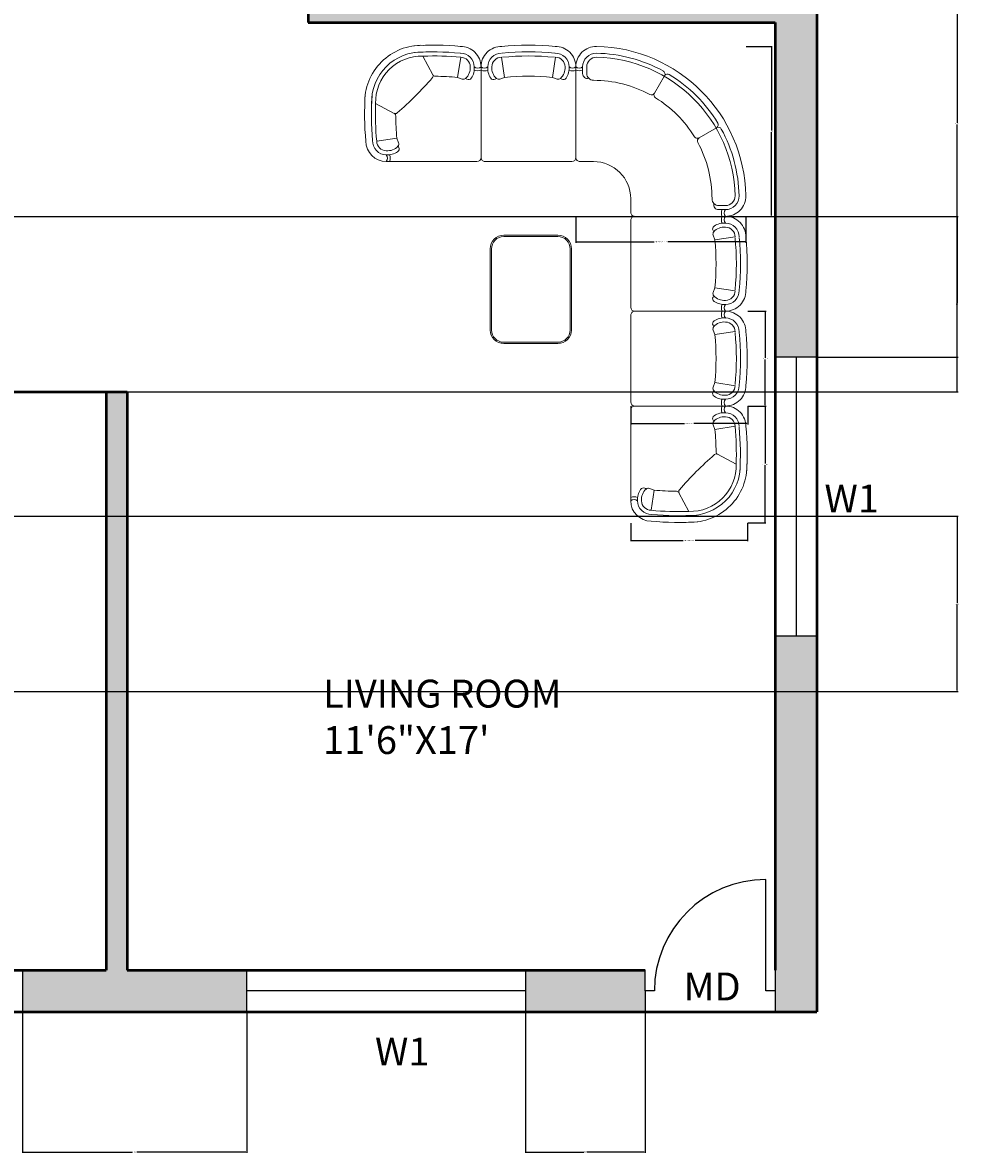
# Model space of a CAD drawing. Units: inches. Extents: x -15 to 420, y -514 to 86.
# Tile 3 of 8: x 218 to 420, y -494 to -251. Entities that reach past the tile are written whole.
import ezdxf

# ---------------------------------------------------------------- set-up
doc = ezdxf.new("R2010")
doc.units = ezdxf.units.IN
doc.header["$MEASUREMENT"] = 0
for name, color, linetype, lineweight in [('A-ANNO-DIMS', 2, 'Continuous', 18), ('A-ANNO-TEXT', 7, 'Continuous', 18), ('A-AREA-IDEN', 7, 'Continuous', 25), ('A-DOOR', 4, 'Continuous', 25), ('A-FURN', 8, 'Continuous', 18), ('A-GLAZ', 41, 'Continuous', 25), ('A-WALL', 7, 'Continuous', 50), ('A-WALL-PATT', 8, 'Continuous', 13)]:
    doc.layers.add(name, color=color, linetype=linetype, lineweight=lineweight)
doc.styles.get("Standard").update_dxf_attribs({"font": 'arial.ttf'})
doc.dimstyles.get("Standard").update_dxf_attribs({"dimtxt": 0.18, "dimasz": 0.18, "dimexe": 0.18, "dimexo": 0.0625, "dimgap": 0.09, "dimtad": 0, "dimtih": 1, "dimtoh": 1, "dimdec": 0, "dimzin": 0, "dimdsep": 46, "dimlunit": 3, "dimtxsty": 'Standard', "dimcen": 0.09, "dimadec": 0, "dimazin": 0, "dimtfac": 1, "dimtdec": 0, "dimtofl": 0, "dimtmove": 0, "dimatfit": 3, "dimfxl": 1, "dimtolj": 1, "dimtzin": 0, "dimarcsym": 0})

# ---------------------------------------------------------------- blocks, each defined once
blk = doc.blocks.new('A$C707258B2')
at = {"color": 0}
for p, q in [((0.4042, 0.342), (1.0739, 0.342)), ((0.4042, 0.292), (0.4544, 0.292)), ((0.4042, 0.262), (0.4539, 0.262)), ((1.1039, 0.312), (1.1039, 0.212)), ((1.4789, -0.063), (1.3789, -0.063)), ((1.5089, -0.7628), (1.5089, -0.093)), ((0.5998, -0.2378), (0.4699, -0.3128)), ((0.9291, -0.5671), (0.8541, -0.697)), ((1.4289, -0.7628), (1.4289, -0.713)), ((1.4589, -0.7628), (1.4589, -0.7125))]:
    blk.add_line(p, q, dxfattribs=at)
for centre, radius, start, end in [((0.4042, 0.192), 0.15, 90, 181.17538), ((0.3779, 0.317), 0.0362, 316.39718, 43.60282), ((0.3679, 0.317), 0.0662, 337.82984, 22.17016), ((1.0739, 0.312), 0.03, 360, 90), ((0.4042, 0.192), 0.1, 90, 181.17538), ((0.4042, 0.192), 0.07, 90, 181.17538), ((0.4539, 0.212), 0.05, 360, 90), ((0.4548, 0.2564), 0.0357, 345.42616, 90.55549), ((1.3789, 0.212), 1.125, 181.17538, 268.82462), ((1.3789, 0.212), 1.075, 181.17538, 208.63569), ((1.3789, 0.212), 1.045, 181.17538, 268.82462), ((1.3789, 0.212), 0.875, 180, 208.40825), ((1.3789, 0.212), 0.275, 180, 270), ((1.4789, -0.093), 0.03, 360, 90), ((0.5873, -0.2162), 0.025, 300, 28.40825), ((0.6123, -0.2595), 0.025, 31.59175, 120), ((1.3789, 0.212), 0.875, 211.59175, 238.40825), ((0.4574, -0.2912), 0.025, 208.63569, 300), ((0.4824, -0.3345), 0.025, 120, 211.36431), ((1.3789, 0.212), 1.075, 211.36431, 238.63569), ((0.9075, -0.5546), 0.025, 330, 58.40825), ((0.9508, -0.5796), 0.025, 61.59175, 150), ((1.3789, 0.212), 0.875, 241.59175, 270), ((1.3789, -0.713), 0.05, 360, 90), ((0.8324, -0.6845), 0.025, 238.63569, 330), ((0.8757, -0.7095), 0.025, 150, 241.36431), ((1.3789, 0.212), 1.075, 241.36431, 268.82462), ((1.4255, -0.7093), 0.0336, 354.63008, 109.38826), ((1.4839, -0.7988), 0.0662, 67.82984, 112.17016), ((1.3589, -0.7628), 0.15, 268.82462, 360), ((1.3589, -0.7628), 0.1, 268.82462, 360), ((1.3589, -0.7628), 0.07, 268.82462, 360), ((1.4839, -0.789), 0.0362, 46.39718, 133.60282)]:
    blk.add_arc(centre, radius, start, end, dxfattribs=at)
blk = doc.blocks.new('part 01')
at = {"color": 0}
for p, q in [((-669.8, 700), (0, 700)), ((30, 30), (30, 670)), ((-590.9, 527.1), (-739.8, 550)), ((-590.9, 527.1), (-578.5, 561.2)), ((-590.9, 172.9), (-739.8, 150)), ((-590.9, 172.9), (-578.5, 138.8)), ((-669.8, 0), (0, 0))]:
    blk.add_line(p, q, dxfattribs=at)
for centre, radius, start, end in [((-669.8, 550), 150, 90, 181.17538), ((-696, 675), 36.2, 316.39718, 43.60282), ((-705.9, 675), 66.2, 337.82984, 22.17016), ((0, 670), 30, 0, 90), ((-669.8, 550), 100, 90, 181.17538), ((-669.8, 550), 70, 90, 181.17538), ((-659.7, 517.8), 132.7, 56.08973, 95.61316), ((-659.7, 517.8), 102.7, 42.00663, 95.61316), ((-599.7, 607.2), 25, 332.96082, 56.08973), ((-624.8, 620), 53.2, 321.00172, 332.96082), ((-602, 569.8), 25, 340, 42.00663), ((1178.1, 350), 2007.9, 174.28354, 185.71646), ((1178.1, 350), 1957.9, 174.28354, 185.71646), ((1178.1, 350), 1927.9, 174.28354, 185.71646), ((1178.1, 350), 1777.9, 174.28354, 185.71646), ((-669.8, 150), 150, 178.82462, 270), ((-669.8, 150), 100, 178.82462, 270), ((-669.8, 150), 70, 178.82462, 270), ((-659.7, 182.2), 102.7, 264.38684, 317.99337), ((-599.7, 92.8), 25, 303.91027, 27.03918), ((-602, 130.2), 25, 317.99337, 20), ((-624.8, 80), 53.2, 27.03918, 38.99828), ((-659.7, 182.2), 132.7, 264.38684, 303.91027), ((-696, 25), 36.2, 316.39718, 43.60282), ((-705.9, 25), 66.2, 337.82984, 22.17016), ((0, 30), 30, 270, 0)]:
    blk.add_arc(centre, radius, start, end, dxfattribs=at)
blk = doc.blocks.new('part02')
at = {"color": 0}
for p, q in [((0, -669.8), (0, 0)), ((30, 30), (699.8, 30)), ((620.9, -142.9), (608.5, -108.8)), ((620.9, -142.9), (769.8, -120)), ((640.4, -325.6), (778.2, -398.9)), ((172.9, -590.9), (138.8, -578.5)), ((172.9, -590.9), (150, -739.8)), ((355.6, -610.4), (428.9, -748.2))]:
    blk.add_line(p, q, dxfattribs=at)
for centre, radius, start, end in [((30, 0), 30, 90, 180), ((726, 5), 56.2, 153.6122, 206.66656), ((726, 5), 36.2, 136.39718, 223.60282), ((699.8, -120), 150, 0, 90), ((629.7, -62.8), 25, 123.91027, 207.03918), ((632, -100.2), 25, 137.99337, 200), ((654.8, -50), 53.2, 207.03918, 218.99828), ((689.7, -152.2), 102.7, 84.38684, 137.99337), ((689.3, -151.3), 131.7, 85.43775, 123.98866), ((699.5, -120.6), 100.6, 357.50055, 89.85796), ((699.8, -120), 70, 0, 90), ((-1148.1, -320), 1777.9, 0.38365, 5.71646), ((-1228.2, -319.5), 2007.9, 357.73494, 5.70316), ((-1148.1, -320), 1957.9, 355.86566, 5.71646), ((-1148.1, -320), 2007.9, 355.81801, 5.71646), ((2219.8, -2189.8), 2454.4, 130.6961, 139.3039), ((632.4, -344.1), 20, 62, 130.6961), ((649.7, -308), 20, 180.38365, 242), ((439.4, -409.4), 418.9, 268.21809, 1.78191), ((439.4, -409.4), 368.9, 268.21809, 1.78191), ((439.4, -409.4), 338.9, 268.21809, 1.78191), ((92.8, -599.7), 25, 62.96082, 146.08973), ((182.2, -659.7), 102.7, 132.00663, 185.61316), ((80, -624.8), 53.2, 51.00172, 62.96082), ((130.2, -602), 25, 70, 132.00663), ((25, -696), 56.2, 63.33344, 116.3878), ((25, -696), 36.2, 46.39718, 133.60282), ((182.2, -659.7), 132.7, 146.08973, 185.61316), ((350, 1178.1), 1777.9, 264.28354, 269.61635), ((338, -619.7), 20, 28, 89.61635), ((374.1, -602.4), 20, 139.3039, 208), ((150, -669.8), 150, 180, 271.17538), ((150, -669.8), 100, 180, 271.17538), ((150, -669.8), 70, 180, 270), ((349.5, 1258.2), 2007.9, 264.29684, 272.26506), ((350, 1178.1), 2007.9, 264.28354, 274.18199), ((350, 1178.1), 1957.9, 264.28354, 274.13434)]:
    blk.add_arc(centre, radius, start, end, dxfattribs=at)
blk = doc.blocks.new('DOOR-SWING-24IN')
for p, q in [((26, 0), (26, 24)), ((2, 0), (0, 0)), ((28, 0), (26, 0))]:
    blk.add_line(p, q)
blk.add_arc((26, 0), 24, 90, 180)
blk = doc.blocks.new('WIN-W1-60IN')
for p, q in [((0, 60), (0, 0)), ((4.5, 60), (4.5, 0)), ((9, 0), (9, 60))]:
    blk.add_line(p, q)
blk = doc.blocks.new('*D25')
at = {"layer": 'A-ANNO-DIMS', "color": 0, "lineweight": -2, "transparency": 16777216}
for p, q in [((349.34, -333.49), (349.34, -337.38)), ((374.51, -333.49), (374.51, -337.38)), ((349.52, -337.2), (360.92, -337.2)), ((374.33, -337.2), (362.92, -337.2))]:
    blk.add_line(p, q, dxfattribs=at)
at = {"layer": 'A-ANNO-DIMS', "color": 0, "transparency": 16777216}
for points in [[(349.52, -337.17), (349.52, -337.23), (349.34, -337.2)], [(374.33, -337.17), (374.33, -337.23), (374.51, -337.2)]]:
    blk.add_solid(points, dxfattribs=at)
at = {"layer": 'Defpoints', "color": 0, "transparency": 16777216}
for p in [(349.34, -333.43), (374.51, -333.43), (349.34, -337.2)]:
    blk.add_point(p, dxfattribs=at)
at = {"layer": 'A-ANNO-DIMS', "color": 0, "transparency": 16777216, "insert": (361.92, -337.2), "char_height": 0.18, "attachment_point": 5}
blk.add_mtext('\\A1;SEAT 2\'-1" TYP.', dxfattribs=at)
blk = doc.blocks.new('*D26')
at = {"layer": 'A-ANNO-DIMS', "color": 0, "lineweight": -2, "transparency": 16777216}
for p, q in [((374.57, -313.02), (378.46, -313.02)), ((378.28, -313.2), (378.28, -323.04)), ((378.28, -333.25), (378.28, -323.41)), ((374.57, -333.43), (378.46, -333.43))]:
    blk.add_line(p, q, dxfattribs=at)
at = {"layer": 'A-ANNO-DIMS', "color": 0, "transparency": 16777216}
for points in [[(378.25, -313.2), (378.31, -313.2), (378.28, -313.02)], [(378.25, -333.25), (378.31, -333.25), (378.28, -333.43)]]:
    blk.add_solid(points, dxfattribs=at)
at = {"layer": 'Defpoints', "color": 0, "transparency": 16777216}
for p in [(374.51, -313.02), (374.51, -333.43), (378.28, -333.43)]:
    blk.add_point(p, dxfattribs=at)
at = {"layer": 'A-ANNO-DIMS', "color": 0, "transparency": 16777216, "insert": (378.28, -323.22), "char_height": 0.18, "attachment_point": 5}
blk.add_mtext('\\A1;1\'-8 1/2" TYP.', dxfattribs=at)
blk = doc.blocks.new('*D27')
at = {"layer": 'A-ANNO-DIMS', "color": 0, "lineweight": -2, "transparency": 16777216}
for p, q in [((349.34, -358.65), (349.34, -362.55)), ((374.5, -358.65), (374.5, -362.55)), ((349.52, -362.37), (360.62, -362.37)), ((374.32, -362.37), (363.21, -362.37))]:
    blk.add_line(p, q, dxfattribs=at)
at = {"layer": 'A-ANNO-DIMS', "color": 0, "transparency": 16777216}
for points in [[(349.52, -362.34), (349.52, -362.4), (349.34, -362.37)], [(374.32, -362.34), (374.32, -362.4), (374.5, -362.37)]]:
    blk.add_solid(points, dxfattribs=at)
at = {"layer": 'Defpoints', "color": 0, "transparency": 16777216}
for p in [(349.34, -358.59), (374.5, -358.59), (349.34, -362.37)]:
    blk.add_point(p, dxfattribs=at)
at = {"layer": 'A-ANNO-DIMS', "color": 0, "transparency": 16777216, "insert": (361.92, -362.37), "char_height": 0.18, "attachment_point": 5}
blk.add_mtext('\\A1;END SEAT 2\'-1" TYP.', dxfattribs=at)
blk = doc.blocks.new('*D28')
at = {"layer": 'A-ANNO-DIMS', "color": 0, "lineweight": -2, "transparency": 16777216}
for p, q in [((374.56, -333.43), (378.45, -333.43)), ((378.27, -333.61), (378.27, -345.83)), ((378.27, -358.41), (378.27, -346.19)), ((374.56, -358.59), (378.45, -358.59))]:
    blk.add_line(p, q, dxfattribs=at)
at = {"layer": 'A-ANNO-DIMS', "color": 0, "transparency": 16777216}
for points in [[(378.24, -333.61), (378.3, -333.61), (378.27, -333.43)], [(378.24, -358.41), (378.3, -358.41), (378.27, -358.59)]]:
    blk.add_solid(points, dxfattribs=at)
at = {"layer": 'Defpoints', "color": 0, "transparency": 16777216}
for p in [(374.5, -333.43), (374.5, -358.59), (378.27, -358.59)]:
    blk.add_point(p, dxfattribs=at)
at = {"layer": 'A-ANNO-DIMS', "color": 0, "transparency": 16777216, "insert": (378.27, -346.01), "char_height": 0.18, "attachment_point": 5}
blk.add_mtext('\\A1;2\'-1" TYP.', dxfattribs=at)
blk = doc.blocks.new('*D29')
at = {"layer": 'A-ANNO-DIMS', "color": 0, "lineweight": -2, "transparency": 16777216}
for p, q in [((337.52, -292.66), (337.52, -298.27)), ((374.14, -292.66), (374.14, -298.27)), ((337.7, -298.09), (354.35, -298.09)), ((373.96, -298.09), (357.31, -298.09))]:
    blk.add_line(p, q, dxfattribs=at)
at = {"layer": 'A-ANNO-DIMS', "color": 0, "transparency": 16777216}
for points in [[(337.7, -298.06), (337.7, -298.12), (337.52, -298.09)], [(373.96, -298.06), (373.96, -298.12), (374.14, -298.09)]]:
    blk.add_solid(points, dxfattribs=at)
at = {"layer": 'Defpoints', "color": 0, "transparency": 16777216}
for p in [(337.52, -292.6), (374.14, -292.6), (337.52, -298.09)]:
    blk.add_point(p, dxfattribs=at)
at = {"layer": 'A-ANNO-DIMS', "color": 0, "transparency": 16777216, "insert": (355.83, -298.09), "char_height": 0.18, "attachment_point": 5}
blk.add_mtext('\\A1;CORNER SEAT 3\'-0 1/2"', dxfattribs=at)
blk = doc.blocks.new('*D30')
at = {"layer": 'A-ANNO-DIMS', "color": 0, "lineweight": -2, "transparency": 16777216}
for p, q in [((374.2, -255.99), (379.81, -255.99)), ((379.63, -256.17), (379.63, -274.11)), ((379.63, -292.42), (379.63, -274.48)), ((374.2, -292.6), (379.81, -292.6))]:
    blk.add_line(p, q, dxfattribs=at)
at = {"layer": 'A-ANNO-DIMS', "color": 0, "transparency": 16777216}
for points in [[(379.6, -256.17), (379.66, -256.17), (379.63, -255.99)], [(379.6, -292.42), (379.66, -292.42), (379.63, -292.6)]]:
    blk.add_solid(points, dxfattribs=at)
at = {"layer": 'Defpoints', "color": 0, "transparency": 16777216}
for p in [(374.14, -255.99), (374.14, -292.6), (379.63, -292.6)]:
    blk.add_point(p, dxfattribs=at)
at = {"layer": 'A-ANNO-DIMS', "color": 0, "transparency": 16777216, "insert": (379.63, -274.29), "char_height": 0.18, "attachment_point": 5}
blk.add_mtext('\\A1;3\'-0 1/2"', dxfattribs=at)
blk = doc.blocks.new('*D47')
at = {"layer": 'A-ANNO-DIMS', "color": 0, "lineweight": -2, "transparency": 16777216}
for p, q in [((164.57, -292.63), (419.8, -292.63)), ((419.62, -292.81), (419.62, -311.32)), ((419.62, -330.2), (419.62, -311.69)), ((164.57, -330.38), (419.8, -330.38))]:
    blk.add_line(p, q, dxfattribs=at)
at = {"layer": 'A-ANNO-DIMS', "color": 0, "transparency": 16777216}
for points in [[(419.59, -292.81), (419.65, -292.81), (419.62, -292.63)], [(419.59, -330.2), (419.65, -330.2), (419.62, -330.38)]]:
    blk.add_solid(points, dxfattribs=at)
at = {"layer": 'Defpoints', "color": 0, "transparency": 16777216}
for p in [(164.51, -292.63), (164.51, -330.38), (419.62, -330.38)]:
    blk.add_point(p, dxfattribs=at)
at = {"layer": 'A-ANNO-DIMS', "color": 0, "transparency": 16777216, "insert": (419.62, -311.5), "char_height": 0.18, "attachment_point": 5}
blk.add_mtext('\\A1;3\'-2"', dxfattribs=at)
blk = doc.blocks.new('*D52')
at = {"layer": 'A-ANNO-DIMS', "color": 0, "lineweight": -2, "transparency": 16777216}
for p, q in [((140.49, -357.15), (419.8, -357.15)), ((419.62, -357.33), (419.62, -375.83)), ((419.62, -394.7), (419.62, -376.2)), ((140.49, -394.88), (419.8, -394.88))]:
    blk.add_line(p, q, dxfattribs=at)
at = {"layer": 'A-ANNO-DIMS', "color": 0, "transparency": 16777216}
for points in [[(419.59, -357.33), (419.65, -357.33), (419.62, -357.15)], [(419.59, -394.7), (419.65, -394.7), (419.62, -394.88)]]:
    blk.add_solid(points, dxfattribs=at)
at = {"layer": 'Defpoints', "color": 0, "transparency": 16777216}
for p in [(140.42, -357.15), (140.42, -394.88), (419.62, -394.88)]:
    blk.add_point(p, dxfattribs=at)
at = {"layer": 'A-ANNO-DIMS', "color": 0, "transparency": 16777216, "insert": (419.62, -376.01), "char_height": 0.18, "attachment_point": 5}
blk.add_mtext('\\A1;3\'-1 1/2"', dxfattribs=at)
blk = doc.blocks.new('*D62')
at = {"layer": 'A-ANNO-DIMS', "color": 0, "lineweight": -2, "transparency": 16777216}
for p, q in [((389.49, -222.38), (419.8, -222.38)), ((419.62, -222.56), (419.62, -272.45)), ((419.62, -322.7), (419.62, -272.81)), ((389.49, -322.88), (419.8, -322.88))]:
    blk.add_line(p, q, dxfattribs=at)
at = {"layer": 'A-ANNO-DIMS', "color": 0, "transparency": 16777216}
for points in [[(419.59, -222.56), (419.65, -222.56), (419.62, -222.38)], [(419.59, -322.7), (419.65, -322.7), (419.62, -322.88)]]:
    blk.add_solid(points, dxfattribs=at)
at = {"layer": 'Defpoints', "color": 0, "transparency": 16777216}
for p in [(389.42, -222.38), (419.62, -222.38), (389.42, -322.88)]:
    blk.add_point(p, dxfattribs=at)
at = {"layer": 'A-ANNO-DIMS', "color": 0, "transparency": 16777216, "insert": (419.62, -272.63), "char_height": 0.18, "attachment_point": 5}
blk.add_mtext('\\A1;8\'-4 1/2"', dxfattribs=at)
blk = doc.blocks.new('*D66')
at = {"layer": 'A-ANNO-DIMS', "color": 0, "lineweight": -2, "transparency": 16777216}
for p, q in [((218.42, -463.94), (218.42, -494.26)), ((266.67, -463.94), (266.67, -494.26)), ((218.6, -494.08), (242.01, -494.08)), ((266.49, -494.08), (243.09, -494.08))]:
    blk.add_line(p, q, dxfattribs=at)
at = {"layer": 'A-ANNO-DIMS', "color": 0, "transparency": 16777216}
for points in [[(218.6, -494.05), (218.6, -494.11), (218.42, -494.08)], [(266.49, -494.05), (266.49, -494.11), (266.67, -494.08)]]:
    blk.add_solid(points, dxfattribs=at)
at = {"layer": 'Defpoints', "color": 0, "transparency": 16777216}
for p in [(218.42, -463.88), (266.67, -463.88), (266.67, -494.08)]:
    blk.add_point(p, dxfattribs=at)
at = {"layer": 'A-ANNO-DIMS', "color": 0, "transparency": 16777216, "insert": (242.55, -494.08), "char_height": 0.18, "attachment_point": 5}
blk.add_mtext('\\A1;4\'-0 1/2"', dxfattribs=at)
blk = doc.blocks.new('*D67')
at = {"layer": 'A-ANNO-DIMS', "color": 0, "lineweight": -2, "transparency": 16777216}
for p, q in [((326.67, -463.94), (326.67, -494.26)), ((352.42, -463.94), (352.42, -494.26)), ((326.85, -494.08), (339.22, -494.08)), ((352.24, -494.08), (339.88, -494.08))]:
    blk.add_line(p, q, dxfattribs=at)
at = {"layer": 'A-ANNO-DIMS', "color": 0, "transparency": 16777216}
for points in [[(326.85, -494.05), (326.85, -494.11), (326.67, -494.08)], [(352.24, -494.05), (352.24, -494.11), (352.42, -494.08)]]:
    blk.add_solid(points, dxfattribs=at)
at = {"layer": 'Defpoints', "color": 0, "transparency": 16777216}
for p in [(326.67, -463.88), (352.42, -463.88), (352.42, -494.08)]:
    blk.add_point(p, dxfattribs=at)
at = {"layer": 'A-ANNO-DIMS', "color": 0, "transparency": 16777216, "insert": (339.55, -494.08), "char_height": 0.18, "attachment_point": 5}
blk.add_mtext('\\A1;2\'-2"', dxfattribs=at)

msp = doc.modelspace()

# ---------------------------------------------------------------- hatches: boundary and pattern name
at = {"layer": 'A-WALL-PATT'}
h = msp.add_hatch(color=256, dxfattribs=at)
h.dxf.hatch_style = 1
h.paths.add_polyline_path([(266.67, -454.88), (240.92, -454.88), (240.92, -330.38), (236.42, -330.38), (236.42, -454.88), (218.42, -454.88), (218.42, -463.88), (266.67, -463.88)])
h.paths.add_polyline_path([(158.42, -454.88), (140.42, -454.88), (140.42, -394.88), (135.92, -394.88), (135.92, -454.88), (39.92, -454.88), (39.92, -412.88), (30.92, -412.88), (30.92, -463.88), (158.42, -463.88)])
h.paths.add_polyline_path([(39.92, -334.88), (135.92, -334.88), (135.92, -357.15), (140.42, -357.15), (140.42, -334.88), (173.95, -334.88), (173.95, -330.38), (39.92, -330.38), (39.92, -250.88), (155.51, -250.88), (155.51, -246.38), (140.42, -246.38), (140.42, -205.38), (138.17, -205.38), (135.92, -205.38), (135.92, -246.38), (39.92, -246.38), (39.92, -222.38), (30.92, -222.38), (30.92, -376.88), (39.92, -376.88)])
h.paths.add_polyline_path([(389.42, -382.88), (380.42, -382.88), (380.42, -454.88), (380.42, -463.88), (389.42, -463.88)])
h.paths.add_polyline_path([(352.42, -459.38), (352.42, -454.88), (326.67, -454.88), (326.67, -463.88), (352.42, -463.88)])
h.paths.add_polyline_path([(176.92, -169.88), (39.92, -169.88), (39.92, -112.88), (30.92, -112.88), (30.92, -198.38), (39.92, -198.38), (39.92, -174.38), (135.92, -174.38), (135.92, -177.38), (140.42, -177.38), (140.42, -174.38), (176.92, -174.38), (176.92, -172.13)])
h.paths.add_polyline_path([(39.92, 4.12), (93.92, 4.12), (93.92, 13.12), (30.92, 13.12), (30.92, -52.88), (39.92, -52.88)])
h.paths.add_polyline_path([(266.42, 13.12), (153.92, 13.12), (153.92, 4.12), (207.92, 4.12), (207.92, -169.88), (204.92, -169.88), (204.92, -174.38), (215.42, -174.38), (215.42, -169.88), (212.42, -169.88), (212.42, 4.12), (266.42, 4.12)])
h.paths.add_polyline_path([(389.42, 13.12), (326.42, 13.12), (326.42, 4.12), (380.42, 4.12), (380.42, -52.88), (389.42, -52.88)])
h.paths.add_polyline_path([(389.42, -112.88), (380.42, -112.88), (380.42, -169.88), (377.42, -169.88), (377.42, -174.38), (380.42, -174.38), (380.42, -198.38), (389.42, -198.38)])
h.paths.add_polyline_path([(349.42, -172.13), (349.42, -169.88), (243.42, -169.88), (243.42, -172.13), (243.42, -174.38), (279.92, -174.38), (279.92, -250.88), (380.42, -250.88), (380.42, -322.88), (389.42, -322.88), (389.42, -222.38), (380.42, -222.38), (380.42, -246.38), (284.42, -246.38), (284.42, -174.38), (349.42, -174.38)])

# ---------------------------------------------------------------- linework, layer by layer
at = {"layer": 'A-DOOR'}
for p, q in [((352.42, -459.38), (352.42, -454.88)), ((380.42, -454.88), (380.42, -463.88)), ((352.42, -459.38), (352.42, -463.88))]:
    msp.add_line(p, q, dxfattribs=at)
at = {"layer": 'A-FURN', "ltscale": 0.03}
for points in [[(333.66, -319.99), (321.99, -319.99, -0.414214), (319.08, -317.07), (319.08, -299.58, -0.414214), (321.99, -296.66), (333.66, -296.66, -0.414214), (336.58, -299.58), (336.58, -317.07, -0.414214)], [(333.66, -319.7), (321.99, -319.7, -0.414214), (319.37, -317.07), (319.37, -299.58, -0.414214), (321.99, -296.95), (333.66, -296.95, -0.414214), (336.28, -299.58), (336.28, -317.07, -0.414214)]]:
    msp.add_lwpolyline(points, format="xyb", close=True, dxfattribs=at)
at = {"layer": 'A-GLAZ'}
for p, q in [((389.42, -322.88), (380.42, -322.88)), ((380.42, -382.88), (389.42, -382.88)), ((218.42, -454.88), (218.42, -463.88)), ((266.67, -463.88), (266.67, -454.88)), ((326.67, -454.88), (326.67, -463.88))]:
    msp.add_line(p, q, dxfattribs=at)
at = {"layer": 'A-WALL'}
for p, q in [((389.42, 13.12), (389.42, -463.88)), ((279.92, -174.38), (279.92, -250.88)), ((279.92, -250.88), (380.42, -250.88)), ((380.42, -250.88), (380.42, -454.88)), ((39.92, -330.38), (240.92, -330.38)), ((236.42, -330.38), (236.42, -454.88)), ((240.92, -330.38), (240.92, -454.88)), ((140.42, -454.88), (236.42, -454.88)), ((240.92, -454.88), (352.42, -454.88)), ((30.92, -463.88), (389.42, -463.88))]:
    msp.add_line(p, q, dxfattribs=at)

# ---------------------------------------------------------------- block references
at = {"layer": 'A-DOOR'}
msp.add_blockref('DOOR-SWING-24IN', (352.42, -459.38), dxfattribs=at)
at = {"layer": 'A-FURN', "ltscale": 0.03}
for name, p, xscale, yscale, zscale, rotation in [('part02', (317.11, -279.92), 0.0291619075652817, 0.0291619075652817, 0.0291619075652817, 180), ('part 01', (317.11, -279.92), 0.0291619075652817, 0.0291619075652817, 0.0291619075652817, 270), ('A$C707258B2', (347.5, -248.6), -29.16190756528171, 29.16190756528171, 29.16190756528171, 89.9999999999967), ('part 01', (350.21, -292.6), 0.0291619075652817, 0.0291619075652817, 0.0291619075652817, 180), ('part 01', (350.21, -313.02), 0.0291619075652817, 0.0291619075652817, 0.0291619075652817, 180), ('part02', (350.21, -333.43), -0.0291619075652817, 0.0291619075652817, 0.0291619075652817, 89.9999999999967)]:
    msp.add_blockref(name, p, dxfattribs=dict(at, xscale=xscale, yscale=yscale, zscale=zscale, rotation=rotation))
at = {"layer": 'A-GLAZ'}
msp.add_blockref('WIN-W1-60IN', (380.43, -382.88), dxfattribs=at)
at = {"layer": 'A-GLAZ', "rotation": 270}
msp.add_blockref('WIN-W1-60IN', (266.68, -454.88), dxfattribs=at)

# ---------------------------------------------------------------- texts
at = {"layer": 'A-ANNO-TEXT', "char_height": 6, "attachment_point": 1}
for s, insert in [('W1', (391.04, -350.35)), ('MD', (360.72, -455.41)), ('W1', (294.28, -469.41))]:
    msp.add_mtext(s, dxfattribs=dict(at, insert=insert))
at = {"layer": 'A-AREA-IDEN', "insert": (283.11, -392.36), "char_height": 6, "attachment_point": 1}
msp.add_mtext('LIVING ROOM\\P11\'6"X17\'', dxfattribs=at)

# ---------------------------------------------------------------- dimensions: what is measured, and where the dimension line sits
at = {"layer": 'A-ANNO-DIMS'}
for base, p1, p2, angle, picture, middle in [((419.62, -222.38), (389.42, -322.88), (389.42, -222.38), 90, '*D62', (419.62, -272.63)), ((379.63, -292.6), (374.14, -255.99), (374.14, -292.6), 270, '*D30', (379.63, -274.29)), ((419.624858, -330.379493), (164.510771, -292.629493), (164.510771, -330.379493), 90, '*D47', (419.624858, -311.504493)), ((419.62, -394.88), (140.42, -357.15), (140.42, -394.88), 90, '*D52', (419.62, -376.01))]:
    dim = msp.add_linear_dim(base=base, p1=p1, p2=p2, angle=angle, dimstyle='Standard', override={"dimdec": 1, "dimlfac": 1, "dimrnd": 0, "dimzin": 1, "dimdsep": 46, "dimlunit": 4, "dimfrac": 2}, dxfattribs=at)
    dim.commit()
    dim.dimension.update_dxf_attribs({"geometry": picture, "text_midpoint": middle})
for base, p1, p2, angle, text, picture, middle in [((337.52, -298.09), (374.14, -292.6), (337.52, -292.6), 180, 'CORNER SEAT <>', '*D29', (355.83, -298.09)), ((378.28, -333.43), (374.51, -313.02), (374.51, -333.43), 270, '<> TYP.', '*D26', (378.28, -323.22)), ((349.34, -337.2), (374.51, -333.43), (349.34, -333.43), 180, 'SEAT <> TYP.', '*D25', (361.92, -337.2)), ((378.27, -358.59), (374.5, -333.43), (374.5, -358.59), 270, '<> TYP.', '*D28', (378.27, -346.01)), ((349.34, -362.37), (374.5, -358.59), (349.34, -358.59), 180, 'END SEAT <> TYP.', '*D27', (361.92, -362.37))]:
    dim = msp.add_linear_dim(base=base, p1=p1, p2=p2, angle=angle, text=text, dimstyle='Standard', override={"dimdec": 1, "dimlfac": 1, "dimrnd": 0, "dimzin": 1, "dimdsep": 46, "dimlunit": 4, "dimfrac": 2}, dxfattribs=at)
    dim.commit()
    dim.dimension.update_dxf_attribs({"geometry": picture, "text_midpoint": middle})
for base, p1, p2, picture, middle in [((266.674858, -494.079493), (218.424858, -463.879493), (266.674858, -463.879493), '*D66', (242.549858, -494.079493)), ((352.424858, -494.079493), (326.674858, -463.879493), (352.424858, -463.879493), '*D67', (339.549858, -494.079493))]:
    dim = msp.add_linear_dim(base=base, p1=p1, p2=p2, dimstyle='Standard', override={"dimdec": 1, "dimlfac": 1, "dimrnd": 0, "dimzin": 1, "dimdsep": 46, "dimlunit": 4, "dimfrac": 2}, dxfattribs=at)
    dim.commit()
    dim.dimension.update_dxf_attribs({"geometry": picture, "text_midpoint": middle})

doc.saveas('drawing.dxf')
